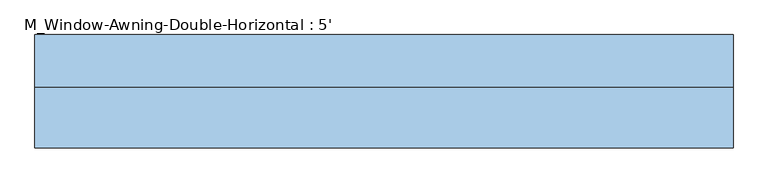
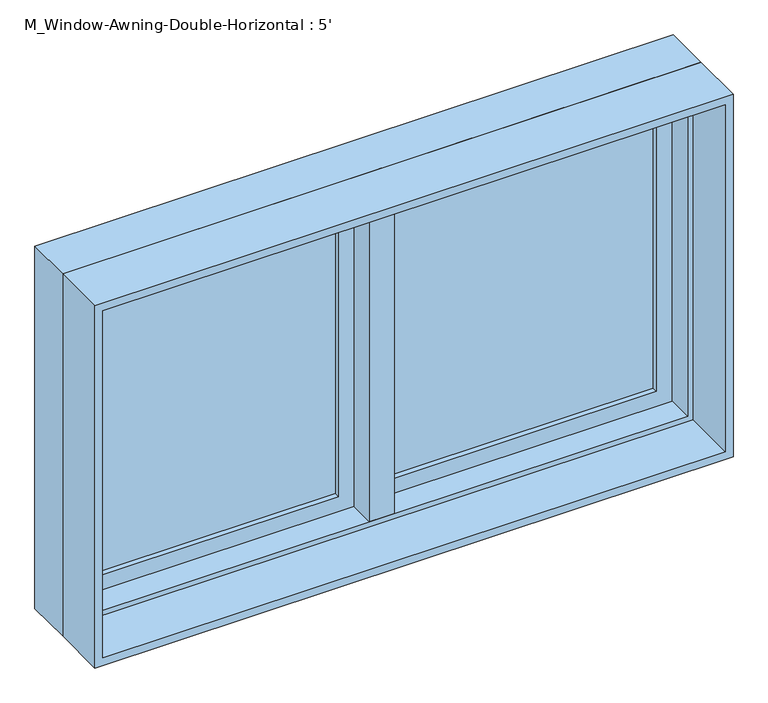
"""IFC4 building model written with IfcOpenShell, lengths in millimetres: window geometry, M_Window-Awning-Double-Horizontal : 5'."""

from ifc_helpers import new_model, si_unit, frame, origin, place, context, project, spatial, polyline, outline, extrude, faceted_brep, source, transform, mapped, element, save


def m_window_awning_double_horizontal_5_7c720334(model_context):
    return source(origin(), model_context, "Body", "SolidModel", [
        faceted_brep([(730.25, 82.55, 1782.65), (730.25, 19.05, 1782.65), (-730.25, 19.05, 1782.65), (-730.25, 82.55, 1782.65), (749.3, 133.35, 1801.7), (749.3, 82.55, 1801.7), (-749.3, 82.55, 1801.7), (-749.3, 133.35, 1801.7), (762.0, 19.05, 1814.4), (762.0, 133.35, 1814.4), (-762.0, 133.35, 1814.4), (-762.0, 19.05, 1814.4), (-730.25, 19.05, 931.75), (-730.25, 82.55, 931.75), (-749.3, 82.55, 912.7), (-749.3, 133.35, 912.7), (-762.0, 133.35, 900.0), (-762.0, 19.05, 900.0), (730.25, 19.05, 931.75), (730.25, 82.55, 931.75), (749.3, 82.55, 912.7), (749.3, 133.35, 912.7), (762.0, 133.35, 900.0), (762.0, 19.05, 900.0)], [[[0, 1, 2, 3]], [[4, 5, 6, 7]], [[8, 9, 10, 11]], [[3, 2, 12, 13]], [[7, 6, 14, 15]], [[11, 10, 16, 17]], [[13, 12, 18, 19]], [[15, 14, 20, 21]], [[17, 16, 22, 23]], [[11, 17, 23, 8], [1, 18, 12, 2]], [[19, 18, 1, 0]], [[5, 20, 14, 6], [3, 13, 19, 0]], [[21, 20, 5, 4]], [[23, 22, 9, 8]], [[9, 22, 16, 10], [7, 15, 21, 4]]]),
        extrude(outline(polyline([(1814.4, -762.0), (900.0, -762.0), (900.0, 762.0), (1814.4, 762.0), (1814.4, -762.0)]), holes=[polyline([(1795.35, 742.95), (919.05, 742.95), (919.05, -742.95), (1795.35, -742.95), (1795.35, 742.95)])]), frame((0.0, -114.3, 0.0), z_axis=(0.0, 1.0, 0.0), x_axis=(0.0, 0.0, 1.0)), (0.0, 0.0, 1.0), 133.35),
        extrude(outline(polyline([(912.7, 749.3), (1801.7, 749.3), (1801.7, 9.525), (912.7, 9.525), (912.7, 749.3)]), holes=[polyline([(969.85, 66.675), (1744.55, 66.675), (1744.55, 692.15), (969.85, 692.15), (969.85, 66.675)])]), frame((0.0, 82.55, 0.0), z_axis=(0.0, 1.0, 0.0), x_axis=(0.0, 0.0, 1.0)), (0.0, 0.0, 1.0), 44.45),
        extrude(outline(polyline([(1801.7, -749.3), (912.7, -749.3), (912.7, -9.525), (1801.7, -9.525), (1801.7, -749.3)]), holes=[polyline([(1744.55, -66.675), (969.85, -66.675), (969.85, -692.15), (1744.55, -692.15), (1744.55, -66.675)])]), frame((0.0, 82.55, 0.0), z_axis=(0.0, 1.0, 0.0), x_axis=(0.0, 0.0, 1.0)), (0.0, 0.0, 1.0), 44.45),
        extrude(outline(polyline([(692.15, 114.3), (692.15, 107.95), (66.675, 107.95), (66.675, 114.3), (692.15, 114.3)])), frame((0.0, 0.0, 969.85), z_axis=(0.0, 0.0, 1.0), x_axis=(1.0, 0.0, 0.0)), (0.0, 0.0, 1.0), 774.7),
        extrude(outline(polyline([(66.675, 95.25), (66.675, 101.6), (692.15, 101.6), (692.15, 95.25), (66.675, 95.25)])), frame((0.0, 0.0, 969.85), z_axis=(0.0, 0.0, 1.0), x_axis=(1.0, 0.0, 0.0)), (0.0, 0.0, 1.0), 774.7),
        extrude(outline(polyline([(-66.675, 114.3), (-66.675, 107.95), (-692.15, 107.95), (-692.15, 114.3), (-66.675, 114.3)])), frame((0.0, 0.0, 969.85), z_axis=(0.0, 0.0, 1.0), x_axis=(1.0, 0.0, 0.0)), (0.0, 0.0, 1.0), 774.7),
        extrude(outline(polyline([(-692.15, 95.25), (-692.15, 101.6), (-66.675, 101.6), (-66.675, 95.25), (-692.15, 95.25)])), frame((0.0, 0.0, 969.85), z_axis=(0.0, 0.0, 1.0), x_axis=(1.0, 0.0, 0.0)), (0.0, 0.0, 1.0), 774.7),
        faceted_brep([(9.525, 133.35, 1801.7), (-9.525, 133.35, 1801.7), (-9.525, 82.55, 1801.7), (9.525, 82.55, 1801.7), (9.525, 133.35, 912.7), (9.525, 82.55, 912.7), (-9.525, 82.55, 912.7), (-9.525, 133.35, 912.7), (-9.525, 82.55, 931.75), (-9.525, 82.55, 1782.65), (-30.1625, 82.55, 931.75), (-30.1625, 82.55, 1782.65), (-30.1625, 19.05, 931.75), (-30.1625, 19.05, 1782.65), (30.1625, 19.05, 931.75), (30.1625, 19.05, 1782.65), (30.1625, 82.55, 931.75), (30.1625, 82.55, 1782.65), (9.525, 82.55, 931.75), (9.525, 82.55, 1782.65)], [[[0, 1, 2, 3]], [[4, 5, 6, 7]], [[1, 0, 4, 7]], [[2, 1, 7, 6, 8, 9]], [[9, 8, 10, 11]], [[11, 10, 12, 13]], [[13, 12, 14, 15]], [[15, 14, 16, 17]], [[17, 16, 18, 19]], [[0, 3, 19, 18, 5, 4]], [[18, 8, 6, 5]], [[9, 19, 3, 2]], [[8, 18, 16, 14, 12, 10]], [[19, 9, 11, 13, 15, 17]]]),
    ])


if __name__ == "__main__":
    model = new_model("IFC4")
    model_context = context("Model", 3, world=origin())
    ifc_project = project(units=[si_unit("LENGTHUNIT", "METRE", prefix="MILLI")], contexts=[model_context])
    site = spatial("IfcSite", under=ifc_project)
    building = spatial("IfcBuilding", under=site)
    placement = place(None, origin())
    m_window_awning_double_horizontal_5_shape = m_window_awning_double_horizontal_5_7c720334(model_context)
    element("IfcWindow", 1, ObjectType="M_Window-Awning-Double-Horizontal : 5'", at=placement, inside=building, context=model_context, shape_type="MappedRepresentation", body=[
        mapped(m_window_awning_double_horizontal_5_shape, transform((0.0, 0.0, 0.0), x_axis=(1.0, 0.0, 0.0), y_axis=(0.0, 1.0, 0.0), z_axis=(0.0, 0.0, 1.0))),
    ])
    save(model, "model.ifc")

# Revit data of these elements
# Type "M_Window-Awning-Double-Horizontal : 5'"
#   Type Mark = "19"
#   Fire Rating = "0.5h"
#   Assembly Code = "B2020100"
#   Analytic Construction = "Double glazing - domestic"
#   Window Inset [instance default] = 0' - 0"
#   Wall Thickness [instance default] = 0' - 5.90551"
#   Interior Wall Closure [instance default] = 0' - 2.15551"
#   Half Width = 2' - 6"
#   Visual Light Transmittance = 0.81
#   Thermal Resistance (R) = 1.8146 (h·ft²·°F)/BTU
#   Solar Heat Gain Coefficient = 0.76
#   Rough Width = 5' - 0.59055"
#   Rough Height = 3' - 0.59055"
#   Height = 3' - 0"
#   Heat Transfer Coefficient (U) = 0.5511 BTU/(h·ft²·°F)
#   Frame Extension [instance default] = 0' - 0 1/4"
#   Exterior Wall Closure [instance default] = 0' - 1 1/4"
#   Extension Jamb [instance default] = 0' - 2.15551"
#   Default Sill Height = 2' - 11.43307"
#   Width = 5' - 0"
#   Muntin Visibility = yes
#   Interior Trim Visibility [instance default] = yes
#   Exterior Trim Visibility [instance default] = yes
#   Extension Jamb Visibility [instance default] = yes
#   Interior Trim Material = Wood - Stained
#   Muntin Pattern = M_Muntin Pattern_2x2 : M_Muntin Pattern_2x2
#   Interior Trim = M_Trim-Window-Interior-Flat : Picture Frame
#   Interior Frame Material = Wood - Stained
#   Glass Panel Material = Glass
#   Exterior Trim Material = Clad - White
#   Exterior Trim = M_Trim-Window-Exterior-Flat : with Sill
#   Exterior Frame Material = Clad - White
#   Wall Closure = (empty or 0)
# Element 1 (IfcWindow, "M_Window-Awning-Double-Horizontal : 5'")
#   Wall Thickness = 0' - 9"
#   Interior Wall Closure = 0' - 2 5/32"
#   Extension Jamb = 0' - 5 1/4"
#   Materials on its faces: "Wood - Stained", "Glass", "Clad - White"
# Materials
#   "Wood - Stained": class "Wood", colour RGB 224 178 126, transparency 0, Cost = 0
#   "Glass": class "Glass", colour RGB 0 128 192, transparency 0.75, Description = "Soda Lime Glass", Cost = 0
#   "Clad - White": class "Wood", colour RGB 242 242 238, transparency 0, Cost = 0
